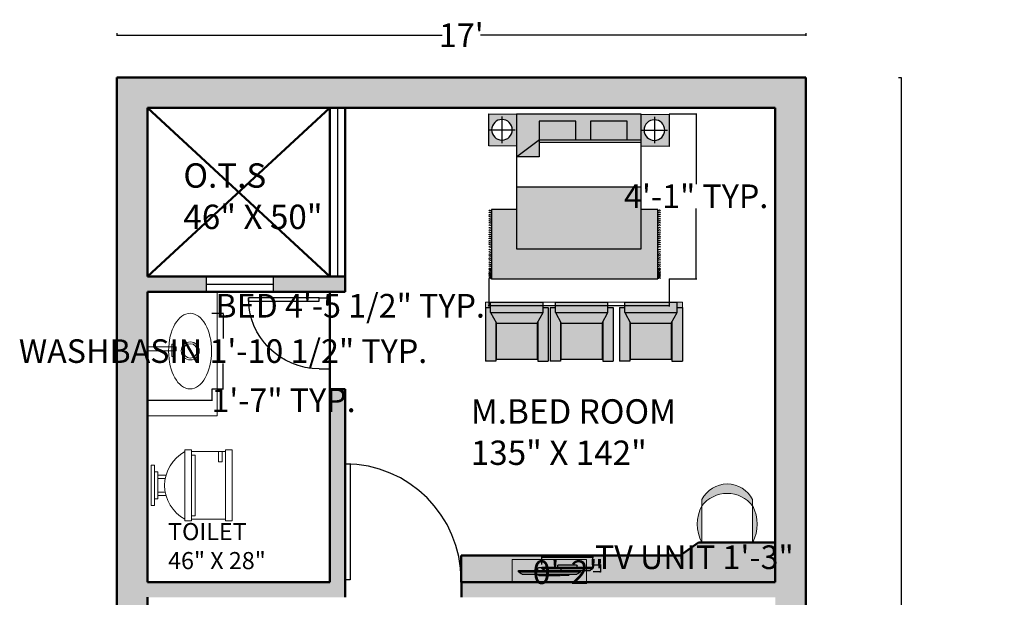
# Model space of a CAD drawing. Units: inches. Extents: x 679 to 1269, y 101 to 755.
# Tile 4 of 6: x 679 to 971, y 584 to 755. Entities that reach past the tile are written whole.
import ezdxf

# ---------------------------------------------------------------- set-up
doc = ezdxf.new("R2010")
doc.units = ezdxf.units.IN
doc.header["$MEASUREMENT"] = 0
for name, color, linetype, lineweight in [('A-ANNO-DIMS', 2, 'Continuous', 18), ('A-AREA-IDEN', 7, 'Continuous', 25), ('A-DOOR', 4, 'Continuous', 25), ('A-FLOR-FIXT', 8, 'Continuous', 18), ('A-FURN', 32, 'Continuous', 18), ('A-FURN-PATT', 252, 'Continuous', 13), ('A-GLAZ', 4, 'Continuous', 25), ('A-WALL', 7, 'Continuous', 50), ('A-WALL-PATT', 8, 'Continuous', 13)]:
    doc.layers.add(name, color=color, linetype=linetype, lineweight=lineweight)
doc.layers.add('furniture', color=32, linetype='Continuous')
doc.styles.get("Standard").update_dxf_attribs({"font": 'arial.ttf'})
doc.dimstyles.get("Standard").update_dxf_attribs({"dimtxt": 7, "dimasz": 0.18, "dimexe": 0.18, "dimexo": 0.0625, "dimgap": 0.09, "dimtad": 0, "dimtih": 1, "dimtoh": 1, "dimzin": 0, "dimdsep": 46, "dimlunit": 3, "dimtxsty": 'Standard', "dimcen": 0.09, "dimadec": 0, "dimazin": 0, "dimtfac": 1, "dimtofl": 0, "dimtmove": 0, "dimatfit": 3, "dimfxl": 1, "dimtolj": 1, "dimtzin": 0, "dimarcsym": 0})

# ---------------------------------------------------------------- blocks, each defined once
blk = doc.blocks.new('*D1')
at = {"layer": 'A-ANNO-DIMS', "color": 0, "lineweight": -2, "transparency": 16777216}
for p, q in [((708.21, 750.86), (708.21, 750.04)), ((708.39, 750.22), (804.51, 750.22)), ((912.03, 750.22), (815.91, 750.22)), ((912.21, 750.86), (912.21, 750.04))]:
    blk.add_line(p, q, dxfattribs=at)
at = {"layer": 'A-ANNO-DIMS', "color": 0, "transparency": 16777216}
for points in [[(708.39, 750.25), (708.39, 750.19), (708.21, 750.22)], [(912.03, 750.25), (912.03, 750.19), (912.21, 750.22)]]:
    blk.add_solid(points, dxfattribs=at)
at = {"layer": 'Defpoints', "color": 0, "transparency": 16777216}
for p in [(708.21, 750.92), (912.21, 750.92), (912.21, 750.22)]:
    blk.add_point(p, dxfattribs=at)
at = {"layer": 'A-ANNO-DIMS', "color": 0, "transparency": 16777216, "insert": (810.21, 750.22), "char_height": 7, "attachment_point": 5}
blk.add_mtext("\\A1;17'", dxfattribs=at)
blk = doc.blocks.new('*D2')
at = {"layer": 'A-ANNO-DIMS', "color": 0, "lineweight": -2, "transparency": 16777216}
for p, q in [((939.65, 737.73), (940.62, 737.73)), ((940.44, 737.55), (940.44, 441.39)), ((940.44, 137.91), (940.44, 434.07)), ((939.65, 137.73), (940.62, 137.73))]:
    blk.add_line(p, q, dxfattribs=at)
at = {"layer": 'A-ANNO-DIMS', "color": 0, "transparency": 16777216}
for points in [[(940.41, 737.55), (940.47, 737.55), (940.44, 737.73)], [(940.41, 137.91), (940.47, 137.91), (940.44, 137.73)]]:
    blk.add_solid(points, dxfattribs=at)
at = {"layer": 'Defpoints', "color": 0, "transparency": 16777216}
for p in [(939.59, 737.73), (939.59, 137.73), (940.44, 137.73)]:
    blk.add_point(p, dxfattribs=at)
at = {"layer": 'A-ANNO-DIMS', "color": 0, "transparency": 16777216, "insert": (940.44, 437.73), "char_height": 7, "attachment_point": 5}
blk.add_mtext("\\A1;50'", dxfattribs=at)
blk = doc.blocks.new('*U4')
for p, q in [((0, 0), (0, -6)), ((40, 0), (40, -6))]:
    blk.add_line(p, q)
blk.add_lwpolyline([(0, 0), (0, 40), (1.75, 40), (1.75, 0)], close=True)
blk.add_arc((0, 0), 40, 0, 90)
blk = doc.blocks.new('CARPET')
at = {"layer": 'furniture'}
for p, q in [((-51.53, -98.11), (-51.53, -55.12)), ((-51.53, -55.12), (-41.27, -55.12)), ((36, -55.12), (51.55, -55.12)), ((51.55, -55.12), (51.55, -98.11)), ((51.55, -98.11), (-51.53, -98.11))]:
    blk.add_line(p, q, dxfattribs=at)
for points, knots in [([(-53.37, -55.99), (-53.22, -55.8), (-52.9, -55.41), (-52.34, -55.8), (-51.89, -56.08), (-51.65, -55.91), (-51.53, -55.83)], [0, 0, 0, 0, 0.653278, 1.290138, 1.740457, 2.114451, 2.114451, 2.114451, 2.114451]), ([(-53.37, -57.26), (-53.22, -57.07), (-52.9, -56.67), (-52.34, -57.07), (-51.89, -57.35), (-51.65, -57.17), (-51.53, -57.1)], [0, 0, 0, 0, 0.653278, 1.290138, 1.740457, 2.114451, 2.114451, 2.114451, 2.114451]), ([(-53.37, -58.59), (-53.22, -58.4), (-52.9, -58.01), (-52.34, -58.4), (-51.89, -58.68), (-51.65, -58.5), (-51.53, -58.43)], [0, 0, 0, 0, 0.653278, 1.290138, 1.740457, 2.114451, 2.114451, 2.114451, 2.114451]), ([(-53.37, -59.78), (-53.22, -59.58), (-52.9, -59.19), (-52.34, -59.58), (-51.89, -59.86), (-51.65, -59.69), (-51.53, -59.61)], [0, 0, 0, 0, 0.653278, 1.290138, 1.740457, 2.114451, 2.114451, 2.114451, 2.114451]), ([(-53.37, -61.22), (-53.22, -61.02), (-52.9, -60.63), (-52.34, -61.02), (-51.89, -61.3), (-51.65, -61.13), (-51.53, -61.05)], [0, 0, 0, 0, 0.653278, 1.290138, 1.740457, 2.114451, 2.114451, 2.114451, 2.114451]), ([(53.37, -55.99), (53.22, -55.8), (52.9, -55.41), (52.34, -55.8), (51.89, -56.08), (51.65, -55.91), (51.53, -55.83)], [0, 0, 0, 0, 0.653278, 1.290138, 1.740457, 2.114451, 2.114451, 2.114451, 2.114451]), ([(53.37, -57.26), (53.22, -57.07), (52.9, -56.67), (52.34, -57.07), (51.89, -57.35), (51.65, -57.17), (51.53, -57.1)], [0, 0, 0, 0, 0.653278, 1.290138, 1.740457, 2.114451, 2.114451, 2.114451, 2.114451]), ([(53.37, -58.59), (53.22, -58.4), (52.9, -58.01), (52.34, -58.4), (51.89, -58.68), (51.65, -58.5), (51.53, -58.43)], [0, 0, 0, 0, 0.653278, 1.290138, 1.740457, 2.114451, 2.114451, 2.114451, 2.114451]), ([(53.37, -59.78), (53.22, -59.58), (52.9, -59.19), (52.34, -59.58), (51.89, -59.86), (51.65, -59.69), (51.53, -59.61)], [0, 0, 0, 0, 0.653278, 1.290138, 1.740457, 2.114451, 2.114451, 2.114451, 2.114451]), ([(53.37, -61.22), (53.22, -61.02), (52.9, -60.63), (52.34, -61.02), (51.89, -61.3), (51.65, -61.13), (51.53, -61.05)], [0, 0, 0, 0, 0.653278, 1.290138, 1.740457, 2.114451, 2.114451, 2.114451, 2.114451]), ([(-53.37, -62.44), (-53.22, -62.25), (-52.9, -61.86), (-52.34, -62.25), (-51.89, -62.53), (-51.65, -62.36), (-51.53, -62.28)], [0, 0, 0, 0, 0.653278, 1.290138, 1.740457, 2.114451, 2.114451, 2.114451, 2.114451]), ([(-53.37, -63.63), (-53.22, -63.43), (-52.9, -63.04), (-52.34, -63.43), (-51.89, -63.72), (-51.65, -63.54), (-51.53, -63.46)], [0, 0, 0, 0, 0.653278, 1.290138, 1.740457, 2.114451, 2.114451, 2.114451, 2.114451]), ([(-53.37, -65.07), (-53.22, -64.87), (-52.9, -64.48), (-52.34, -64.87), (-51.89, -65.15), (-51.65, -64.98), (-51.53, -64.9)], [0, 0, 0, 0, 0.653278, 1.290138, 1.740457, 2.114451, 2.114451, 2.114451, 2.114451]), ([(-53.37, -66.76), (-53.22, -66.56), (-52.9, -66.17), (-52.34, -66.56), (-51.89, -66.84), (-51.65, -66.67), (-51.53, -66.59)], [0, 0, 0, 0, 0.653278, 1.290138, 1.740457, 2.114451, 2.114451, 2.114451, 2.114451]), ([(53.37, -62.44), (53.22, -62.25), (52.9, -61.86), (52.34, -62.25), (51.89, -62.53), (51.65, -62.36), (51.53, -62.28)], [0, 0, 0, 0, 0.653278, 1.290138, 1.740457, 2.114451, 2.114451, 2.114451, 2.114451]), ([(53.37, -63.63), (53.22, -63.43), (52.9, -63.04), (52.34, -63.43), (51.89, -63.72), (51.65, -63.54), (51.53, -63.46)], [0, 0, 0, 0, 0.653278, 1.290138, 1.740457, 2.114451, 2.114451, 2.114451, 2.114451]), ([(53.37, -65.07), (53.22, -64.87), (52.9, -64.48), (52.34, -64.87), (51.89, -65.15), (51.65, -64.98), (51.53, -64.9)], [0, 0, 0, 0, 0.653278, 1.290138, 1.740457, 2.114451, 2.114451, 2.114451, 2.114451]), ([(53.37, -66.76), (53.22, -66.56), (52.9, -66.17), (52.34, -66.56), (51.89, -66.84), (51.65, -66.67), (51.53, -66.59)], [0, 0, 0, 0, 0.653278, 1.290138, 1.740457, 2.114451, 2.114451, 2.114451, 2.114451]), ([(-53.37, -68.2), (-53.22, -68), (-52.9, -67.61), (-52.34, -68), (-51.89, -68.28), (-51.65, -68.11), (-51.53, -68.03)], [0, 0, 0, 0, 0.653278, 1.290138, 1.740457, 2.114451, 2.114451, 2.114451, 2.114451]), ([(-53.37, -69.53), (-53.22, -69.33), (-52.9, -68.94), (-52.34, -69.33), (-51.89, -69.61), (-51.65, -69.44), (-51.53, -69.36)], [0, 0, 0, 0, 0.653278, 1.290138, 1.740457, 2.114451, 2.114451, 2.114451, 2.114451]), ([(-53.37, -70.79), (-53.22, -70.6), (-52.9, -70.21), (-52.34, -70.6), (-51.89, -70.88), (-51.65, -70.7), (-51.53, -70.63)], [0, 0, 0, 0, 0.653278, 1.290138, 1.740457, 2.114451, 2.114451, 2.114451, 2.114451]), ([(-53.37, -72.12), (-53.22, -71.93), (-52.9, -71.54), (-52.34, -71.93), (-51.89, -72.21), (-51.65, -72.04), (-51.53, -71.96)], [0, 0, 0, 0, 0.653278, 1.290138, 1.740457, 2.114451, 2.114451, 2.114451, 2.114451]), ([(-53.37, -73.31), (-53.22, -73.11), (-52.9, -72.72), (-52.34, -73.11), (-51.89, -73.4), (-51.65, -73.22), (-51.53, -73.14)], [0, 0, 0, 0, 0.653278, 1.290138, 1.740457, 2.114451, 2.114451, 2.114451, 2.114451]), ([(53.37, -68.2), (53.22, -68), (52.9, -67.61), (52.34, -68), (51.89, -68.28), (51.65, -68.11), (51.53, -68.03)], [0, 0, 0, 0, 0.653278, 1.290138, 1.740457, 2.114451, 2.114451, 2.114451, 2.114451]), ([(53.37, -69.53), (53.22, -69.33), (52.9, -68.94), (52.34, -69.33), (51.89, -69.61), (51.65, -69.44), (51.53, -69.36)], [0, 0, 0, 0, 0.653278, 1.290138, 1.740457, 2.114451, 2.114451, 2.114451, 2.114451]), ([(53.37, -70.79), (53.22, -70.6), (52.9, -70.21), (52.34, -70.6), (51.89, -70.88), (51.65, -70.7), (51.53, -70.63)], [0, 0, 0, 0, 0.653278, 1.290138, 1.740457, 2.114451, 2.114451, 2.114451, 2.114451]), ([(53.37, -72.12), (53.22, -71.93), (52.9, -71.54), (52.34, -71.93), (51.89, -72.21), (51.65, -72.04), (51.53, -71.96)], [0, 0, 0, 0, 0.653278, 1.290138, 1.740457, 2.114451, 2.114451, 2.114451, 2.114451]), ([(53.37, -73.31), (53.22, -73.11), (52.9, -72.72), (52.34, -73.11), (51.89, -73.4), (51.65, -73.22), (51.53, -73.14)], [0, 0, 0, 0, 0.653278, 1.290138, 1.740457, 2.114451, 2.114451, 2.114451, 2.114451]), ([(-53.37, -74.75), (-53.22, -74.55), (-52.9, -74.16), (-52.34, -74.55), (-51.89, -74.83), (-51.65, -74.66), (-51.53, -74.58)], [0, 0, 0, 0, 0.653278, 1.290138, 1.740457, 2.114451, 2.114451, 2.114451, 2.114451]), ([(-53.37, -75.98), (-53.22, -75.78), (-52.9, -75.39), (-52.34, -75.78), (-51.89, -76.06), (-51.65, -75.89), (-51.53, -75.81)], [0, 0, 0, 0, 0.653278, 1.290138, 1.740457, 2.114451, 2.114451, 2.114451, 2.114451]), ([(-53.37, -77.16), (-53.22, -76.96), (-52.9, -76.57), (-52.34, -76.96), (-51.89, -77.25), (-51.65, -77.07), (-51.53, -76.99)], [0, 0, 0, 0, 0.653278, 1.290138, 1.740457, 2.114451, 2.114451, 2.114451, 2.114451]), ([(-53.37, -78.6), (-53.22, -78.4), (-52.9, -78.01), (-52.34, -78.4), (-51.89, -78.68), (-51.65, -78.51), (-51.53, -78.43)], [0, 0, 0, 0, 0.653278, 1.290138, 1.740457, 2.114451, 2.114451, 2.114451, 2.114451]), ([(53.37, -74.75), (53.22, -74.55), (52.9, -74.16), (52.34, -74.55), (51.89, -74.83), (51.65, -74.66), (51.53, -74.58)], [0, 0, 0, 0, 0.653278, 1.290138, 1.740457, 2.114451, 2.114451, 2.114451, 2.114451]), ([(53.37, -75.98), (53.22, -75.78), (52.9, -75.39), (52.34, -75.78), (51.89, -76.06), (51.65, -75.89), (51.53, -75.81)], [0, 0, 0, 0, 0.653278, 1.290138, 1.740457, 2.114451, 2.114451, 2.114451, 2.114451]), ([(53.37, -77.16), (53.22, -76.96), (52.9, -76.57), (52.34, -76.96), (51.89, -77.25), (51.65, -77.07), (51.53, -76.99)], [0, 0, 0, 0, 0.653278, 1.290138, 1.740457, 2.114451, 2.114451, 2.114451, 2.114451]), ([(53.37, -78.6), (53.22, -78.4), (52.9, -78.01), (52.34, -78.4), (51.89, -78.68), (51.65, -78.51), (51.53, -78.43)], [0, 0, 0, 0, 0.653278, 1.290138, 1.740457, 2.114451, 2.114451, 2.114451, 2.114451]), ([(-53.37, -80.29), (-53.22, -80.09), (-52.9, -79.7), (-52.34, -80.09), (-51.89, -80.37), (-51.65, -80.2), (-51.53, -80.12)], [0, 0, 0, 0, 0.653278, 1.290138, 1.740457, 2.114451, 2.114451, 2.114451, 2.114451]), ([(-53.37, -81.73), (-53.22, -81.53), (-52.9, -81.14), (-52.34, -81.53), (-51.89, -81.81), (-51.65, -81.64), (-51.53, -81.56)], [0, 0, 0, 0, 0.653278, 1.290138, 1.740457, 2.114451, 2.114451, 2.114451, 2.114451]), ([(-53.37, -83.06), (-53.22, -82.86), (-52.9, -82.47), (-52.34, -82.86), (-51.89, -83.14), (-51.65, -82.97), (-51.53, -82.89)], [0, 0, 0, 0, 0.653278, 1.290138, 1.740457, 2.114451, 2.114451, 2.114451, 2.114451]), ([(-53.37, -84.18), (-53.22, -83.99), (-52.9, -83.6), (-52.34, -83.99), (-51.89, -84.27), (-51.65, -84.09), (-51.53, -84.02)], [0, 0, 0, 0, 0.653278, 1.290138, 1.740457, 2.114451, 2.114451, 2.114451, 2.114451]), ([(-53.37, -85.51), (-53.22, -85.32), (-52.9, -84.93), (-52.34, -85.32), (-51.89, -85.6), (-51.65, -85.42), (-51.53, -85.35)], [0, 0, 0, 0, 0.653278, 1.290138, 1.740457, 2.114451, 2.114451, 2.114451, 2.114451]), ([(53.37, -80.29), (53.22, -80.09), (52.9, -79.7), (52.34, -80.09), (51.89, -80.37), (51.65, -80.2), (51.53, -80.12)], [0, 0, 0, 0, 0.653278, 1.290138, 1.740457, 2.114451, 2.114451, 2.114451, 2.114451]), ([(53.37, -81.73), (53.22, -81.53), (52.9, -81.14), (52.34, -81.53), (51.89, -81.81), (51.65, -81.64), (51.53, -81.56)], [0, 0, 0, 0, 0.653278, 1.290138, 1.740457, 2.114451, 2.114451, 2.114451, 2.114451]), ([(53.37, -83.06), (53.22, -82.86), (52.9, -82.47), (52.34, -82.86), (51.89, -83.14), (51.65, -82.97), (51.53, -82.89)], [0, 0, 0, 0, 0.653278, 1.290138, 1.740457, 2.114451, 2.114451, 2.114451, 2.114451]), ([(53.37, -84.18), (53.22, -83.99), (52.9, -83.6), (52.34, -83.99), (51.89, -84.27), (51.65, -84.09), (51.53, -84.02)], [0, 0, 0, 0, 0.653278, 1.290138, 1.740457, 2.114451, 2.114451, 2.114451, 2.114451]), ([(53.37, -85.51), (53.22, -85.32), (52.9, -84.93), (52.34, -85.32), (51.89, -85.6), (51.65, -85.42), (51.53, -85.35)], [0, 0, 0, 0, 0.653278, 1.290138, 1.740457, 2.114451, 2.114451, 2.114451, 2.114451]), ([(-53.37, -86.7), (-53.22, -86.5), (-52.9, -86.11), (-52.34, -86.5), (-51.89, -86.78), (-51.65, -86.61), (-51.53, -86.53)], [0, 0, 0, 0, 0.653278, 1.290138, 1.740457, 2.114451, 2.114451, 2.114451, 2.114451]), ([(-53.37, -88.14), (-53.22, -87.94), (-52.9, -87.55), (-52.34, -87.94), (-51.89, -88.22), (-51.65, -88.05), (-51.53, -87.97)], [0, 0, 0, 0, 0.653278, 1.290138, 1.740457, 2.114451, 2.114451, 2.114451, 2.114451]), ([(-53.37, -89.36), (-53.22, -89.17), (-52.9, -88.78), (-52.34, -89.17), (-51.89, -89.45), (-51.65, -89.28), (-51.53, -89.2)], [0, 0, 0, 0, 0.653278, 1.290138, 1.740457, 2.114451, 2.114451, 2.114451, 2.114451]), ([(-53.37, -90.55), (-53.22, -90.35), (-52.9, -89.96), (-52.34, -90.35), (-51.89, -90.64), (-51.65, -90.46), (-51.53, -90.38)], [0, 0, 0, 0, 0.653278, 1.290138, 1.740457, 2.114451, 2.114451, 2.114451, 2.114451]), ([(-53.37, -91.99), (-53.22, -91.79), (-52.9, -91.4), (-52.34, -91.79), (-51.89, -92.07), (-51.65, -91.9), (-51.53, -91.82)], [0, 0, 0, 0, 0.653278, 1.290138, 1.740457, 2.114451, 2.114451, 2.114451, 2.114451]), ([(53.37, -86.7), (53.22, -86.5), (52.9, -86.11), (52.34, -86.5), (51.89, -86.78), (51.65, -86.61), (51.53, -86.53)], [0, 0, 0, 0, 0.653278, 1.290138, 1.740457, 2.114451, 2.114451, 2.114451, 2.114451]), ([(53.37, -88.14), (53.22, -87.94), (52.9, -87.55), (52.34, -87.94), (51.89, -88.22), (51.65, -88.05), (51.53, -87.97)], [0, 0, 0, 0, 0.653278, 1.290138, 1.740457, 2.114451, 2.114451, 2.114451, 2.114451]), ([(53.37, -89.36), (53.22, -89.17), (52.9, -88.78), (52.34, -89.17), (51.89, -89.45), (51.65, -89.28), (51.53, -89.2)], [0, 0, 0, 0, 0.653278, 1.290138, 1.740457, 2.114451, 2.114451, 2.114451, 2.114451]), ([(53.37, -90.55), (53.22, -90.35), (52.9, -89.96), (52.34, -90.35), (51.9, -90.63), (51.66, -90.47), (51.55, -90.4)], [0, 0, 0, 0, 0.653278, 1.290138, 1.740457, 2.0926, 2.0926, 2.0926, 2.0926]), ([(53.37, -91.99), (53.22, -91.79), (52.9, -91.4), (52.34, -91.79), (51.9, -92.07), (51.66, -91.91), (51.55, -91.83)], [0, 0, 0, 0, 0.653278, 1.290138, 1.740457, 2.0926, 2.0926, 2.0926, 2.0926]), ([(-53.37, -92.69), (-53.22, -92.48), (-52.9, -92.08), (-52.35, -92.49), (-51.89, -92.77), (-51.65, -92.6), (-51.53, -92.52)], [0, 0, 0, 0, 0.663904, 1.307406, 1.757725, 2.131719, 2.131719, 2.131719, 2.131719]), ([(-53.37, -93.61), (-53.22, -93.42), (-52.9, -93.03), (-52.34, -93.42), (-51.89, -93.7), (-51.65, -93.52), (-51.53, -93.45)], [0, 0, 0, 0, 0.653278, 1.290138, 1.740457, 2.114451, 2.114451, 2.114451, 2.114451]), ([(-53.37, -94.55), (-53.22, -94.35), (-52.9, -93.96), (-52.34, -94.35), (-51.89, -94.63), (-51.65, -94.46), (-51.53, -94.38)], [0, 0, 0, 0, 0.653278, 1.290138, 1.740457, 2.114451, 2.114451, 2.114451, 2.114451]), ([(-53.37, -95.05), (-53.22, -94.85), (-52.9, -94.46), (-52.34, -94.85), (-51.89, -95.14), (-51.65, -94.96), (-51.53, -94.88)], [0, 0, 0, 0, 0.653278, 1.290138, 1.740457, 2.114451, 2.114451, 2.114451, 2.114451]), ([(-53.37, -95.73), (-53.22, -95.54), (-52.9, -95.15), (-52.34, -95.54), (-51.89, -95.82), (-51.65, -95.65), (-51.53, -95.57)], [0, 0, 0, 0, 0.653278, 1.290138, 1.740457, 2.114451, 2.114451, 2.114451, 2.114451]), ([(-53.37, -96.38), (-53.22, -96.18), (-52.9, -95.79), (-52.34, -96.18), (-51.89, -96.47), (-51.65, -96.29), (-51.53, -96.21)], [0, 0, 0, 0, 0.653278, 1.290138, 1.740457, 2.114451, 2.114451, 2.114451, 2.114451]), ([(-53.37, -97.17), (-53.22, -96.98), (-52.9, -96.59), (-52.34, -96.98), (-51.89, -97.26), (-51.65, -97.08), (-51.53, -97.01)], [0, 0, 0, 0, 0.653278, 1.290138, 1.740457, 2.114451, 2.114451, 2.114451, 2.114451]), ([(-53.37, -97.99), (-53.22, -97.79), (-52.9, -97.4), (-52.34, -97.79), (-51.89, -98.08), (-51.65, -97.9), (-51.53, -97.82)], [0, 0, 0, 0, 0.653278, 1.290138, 1.740457, 2.114451, 2.114451, 2.114451, 2.114451]), ([(53.37, -95.78), (53.22, -95.58), (52.9, -95.19), (52.34, -95.58), (51.89, -95.86), (51.65, -95.69), (51.53, -95.61)], [0, 0, 0, 0, 0.653278, 1.290138, 1.740457, 2.114451, 2.114451, 2.114451, 2.114451]), ([(53.37, -96.43), (53.22, -96.23), (52.9, -95.84), (52.34, -96.23), (51.89, -96.51), (51.65, -96.34), (51.53, -96.26)], [0, 0, 0, 0, 0.653278, 1.290138, 1.740457, 2.114451, 2.114451, 2.114451, 2.114451]), ([(53.37, -97.22), (53.22, -97.02), (52.9, -96.63), (52.34, -97.02), (51.89, -97.3), (51.65, -97.13), (51.53, -97.05)], [0, 0, 0, 0, 0.653278, 1.290138, 1.740457, 2.114451, 2.114451, 2.114451, 2.114451]), ([(53.37, -97.99), (53.22, -97.79), (52.9, -97.4), (52.34, -97.79), (51.89, -98.08), (51.65, -97.9), (51.53, -97.82)], [0, 0, 0, 0, 0.653278, 1.290138, 1.740457, 2.114451, 2.114451, 2.114451, 2.114451]), ([(53.37, -92.69), (53.22, -92.49), (52.9, -92.09), (52.34, -92.49), (51.9, -92.77), (51.66, -92.61), (51.55, -92.53)], [0, 0, 0, 0, 0.656792, 1.295826, 1.746145, 2.098292, 2.098292, 2.098292, 2.098292]), ([(53.37, -93.66), (53.22, -93.46), (52.9, -93.07), (52.34, -93.46), (51.9, -93.74), (51.66, -93.58), (51.55, -93.5)], [0, 0, 0, 0, 0.653278, 1.290138, 1.740457, 2.0926, 2.0926, 2.0926, 2.0926]), ([(53.37, -94.59), (53.22, -94.4), (52.9, -94.01), (52.34, -94.4), (51.9, -94.68), (51.66, -94.51), (51.55, -94.44)], [0, 0, 0, 0, 0.653278, 1.290138, 1.740457, 2.0926, 2.0926, 2.0926, 2.0926]), ([(53.37, -95.1), (53.22, -94.9), (52.9, -94.51), (52.34, -94.9), (51.9, -95.18), (51.66, -95.02), (51.55, -94.94)], [0, 0, 0, 0, 0.653278, 1.290138, 1.740457, 2.0926, 2.0926, 2.0926, 2.0926])]:
    blk.add_open_spline(points, degree=3, knots=knots, dxfattribs=at)
blk = doc.blocks.new('A$C58D270C6')
at = {"layer": 'furniture'}
for p, q in [((9.09, 124.13), (9.09, 108.87)), ((1.46, 116.5), (16.73, 116.5)), ((14.97, 94.84), (24.62, 107.92)), ((24.62, 94.93), (24.62, 107.92)), ((42.08, 108), (42.08, 36)), ((14.97, 94.93), (24.62, 94.93)), ((14.97, 94.84), (14.97, 36)), ((16.22, 94.93), (16.22, 36)), ((9.25, 36), (9.25, 20.74)), ((1.62, 28.37), (16.88, 28.37))]:
    blk.add_line(p, q, dxfattribs=at)
for points in [[(18.5, 108), (18.34, 124.13), (-0.16, 124.13), (0, 108)], [(0, 108), (77.91, 108), (77.91, 36), (0, 36)], [(4.09, 94.93), (14.97, 94.93), (14.97, 73.83), (4.09, 73.83)], [(4.09, 65.23), (14.97, 65.23), (14.97, 44.13), (4.09, 44.13)], [(18.65, 19.87), (18.5, 36), (0, 36), (0.16, 19.87)]]:
    blk.add_lwpolyline(points, close=True, dxfattribs=at)
for centre in [(9.09, 116.5), (9.25, 28.37)]:
    blk.add_circle(centre, 5.95, dxfattribs=at)
at = {"layer": 'furniture', "xscale": 0.9312884925094044, "yscale": 0.9312884925094044, "zscale": 0.9312884925094044, "rotation": 90}
blk.add_blockref('CARPET', (3.79, 74.47), dxfattribs=at)
blk = doc.blocks.new('FABRIC SOFA 1S')
at = {"layer": 'furniture'}
for p, q in [((3, 18.12), (34, 18.12)), ((3, 15.12), (3, 18.12)), ((34, 12.12), (34, 18.12)), ((0, -15.12), (0, 15.12)), ((6, 15.12), (0, 15.12)), ((6, -15.12), (6, 15.12)), ((12, 11.75), (6, 15.12)), ((11.33, 12.12), (34, 12.12)), ((6, -15.12), (0, -15.12)), ((3, -18.12), (3, -15.12)), ((6, -15.12), (12, -11.75)), ((11.33, -12.12), (34, -12.12)), ((34, -12.12), (34, -18.12)), ((3, -18.12), (34, -18.12))]:
    blk.add_line(p, q, dxfattribs=at)
blk.add_lwpolyline([(12, -11.75), (12, 11.75), (33, 11.75), (33, -11.75)], close=True, dxfattribs=at)
blk = doc.blocks.new('*U12')
for p, q in [((-10, 22), (-10, 12)), ((-10, 21), (-7, 21)), ((-7, 21), (-7, 20)), ((10, 12), (10, 22)), ((-7, 20), (-10, 20)), ((10.5, 12), (-10.5, 12)), ((-10.5, 10), (-10.5, 12)), ((9, 13), (-9, 13)), ((-9, 13), (-9, 12)), ((9, 12), (9, 13)), ((10.5, 12), (10.5, 10)), ((10.5, 10), (-10.5, 10)), ((-3, 4.4065), (-3, 2)), ((-2, 2), (-2, 4.1658)), ((2, 4.1658), (2, 2)), ((3, 2), (3, 4.4065)), ((4, 2), (-4, 2)), ((-4, 2), (-4, 1)), ((4, 1), (4, 2))]:
    blk.add_line(p, q)
for points in [[(10.5, 22), (10.5, 24), (-10.5, 24), (-10.5, 22)], [(6, 0), (6, 1), (-6, 1), (-6, 0)]]:
    blk.add_lwpolyline(points, close=True)
blk.add_arc((0, 15.3333), 11.3333, 208.0725, 331.9275)
blk = doc.blocks.new('PLASMA-LARGE')
at = {"layer": 'furniture'}
for p, q in [((-7.26, 0), (7.26, 0)), ((-21, -2.5), (21, -2.5)), ((-21, -2.5), (-21, -3.5)), ((-21, -3.5), (21, -3.5)), ((-18.61, -1), (18.61, -1)), ((-8, -1), (-8, -0.74)), ((-8, -3.5), (-8, -4.76)), ((-7.26, -5.5), (7.26, -5.5)), ((8, -1), (8, -0.74)), ((8, -3.5), (8, -4.76)), ((21, -2.5), (21, -3.5))]:
    blk.add_line(p, q, dxfattribs=at)
for centre, radius, start, end in [((-7.26, -0.74), 0.744, 90, 180), ((7.26, -0.74), 0.744, 0, 90), ((-13.97, -11.05), 11.07, 114.76019, 129.41749), ((-7.26, -4.76), 0.744, 180, 270), ((7.26, -4.76), 0.744, 270, 0), ((13.97, -11.05), 11.07, 50.58251, 65.23981)]:
    blk.add_arc(centre, radius, start, end, dxfattribs=at)
blk = doc.blocks.new('WASHBASIN')
for p, q in [((8.57, 12.49), (0, 12.49)), ((7.24, 9.62), (7.23, 13.28)), ((7.23, 13.28), (7.63, 13.28)), ((7.63, 13.28), (7.65, 9.63)), ((8.57, 11.25), (8.57, 12.49)), ((8.57, 11.25), (0, 11.25)), ((7.24, 9.62), (7.65, 9.63))]:
    blk.add_line(p, q)
for radius in [2.67, 2.13]:
    blk.add_circle((12.7, 11.27), radius)
at = {"extrusion": (0, 0, -1)}
blk.add_ellipse((12.66, 11.2), major_axis=(0.03, 11.2), ratio=0.56899, dxfattribs=at)
blk = doc.blocks.new('CHAIR')
h = blk.add_hatch(color=256)
h.dxf.hatch_style = 1
h.paths.add_polyline_path([(1.35, 12.72), (1.35, 10.82, -0.490483), (16.4, 10.82), (16.4, 12.72, 0.611129)])
h.paths.add_polyline_path([(1.35, 10.82, 0.248963), (1.35, 0)])
h.paths.add_polyline_path([(16.4, 10.82), (16.4, 0, 0.248963)])
for p, q in [((1.35, 12.72), (1.35, 0)), ((16.4, 12.72), (16.4, 0))]:
    blk.add_line(p, q)
for centre, radius, start, end in [((8.87, 8.86), 8.46, 27.1394, 152.8606), ((8.87, 4.99), 9.52, 37.7457, 142.2543), ((11.54, 5.41), 11.54, 152.0394, 207.9606), ((6.21, 5.41), 11.54, 332.0394, 27.9606)]:
    blk.add_arc(centre, radius, start, end)
blk = doc.blocks.new('*D21')
at = {"layer": 'A-ANNO-DIMS', "color": 0, "lineweight": -2, "transparency": 16777216}
for p, q in [((818.31, 678.03), (818.31, 669.9)), ((871.75, 678.03), (871.75, 669.9)), ((818.31, 670.08), (818.13, 670.08)), ((871.57, 670.08), (818.49, 670.08))]:
    blk.add_line(p, q, dxfattribs=at)
at = {"layer": 'A-ANNO-DIMS', "color": 0, "transparency": 16777216}
for points in [[(818.49, 670.11), (818.49, 670.05), (818.31, 670.08)], [(871.57, 670.11), (871.57, 670.05), (871.75, 670.08)]]:
    blk.add_solid(points, dxfattribs=at)
at = {"layer": 'Defpoints', "color": 0, "transparency": 16777216}
for p in [(818.31, 678.1), (871.75, 678.1), (818.31, 670.08)]:
    blk.add_point(p, dxfattribs=at)
at = {"layer": 'A-ANNO-DIMS', "color": 0, "transparency": 16777216, "insert": (777.29, 670.08), "char_height": 7, "attachment_point": 5}
blk.add_mtext('\\A1;BED 4\'-5 1/2" TYP.', dxfattribs=at)
blk = doc.blocks.new('*D22')
at = {"layer": 'A-ANNO-DIMS', "color": 0, "lineweight": -2, "transparency": 16777216}
for p, q in [((871.81, 726.93), (879.95, 726.93)), ((879.77, 726.75), (879.77, 706.12)), ((879.77, 678.28), (879.77, 698.91)), ((871.81, 678.1), (879.95, 678.1))]:
    blk.add_line(p, q, dxfattribs=at)
at = {"layer": 'A-ANNO-DIMS', "color": 0, "transparency": 16777216}
for points in [[(879.74, 726.75), (879.8, 726.75), (879.77, 726.93)], [(879.74, 678.28), (879.8, 678.28), (879.77, 678.1)]]:
    blk.add_solid(points, dxfattribs=at)
at = {"layer": 'Defpoints', "color": 0, "transparency": 16777216}
for p in [(871.75, 726.93), (871.75, 678.1), (879.77, 678.1)]:
    blk.add_point(p, dxfattribs=at)
at = {"layer": 'A-ANNO-DIMS', "color": 0, "transparency": 16777216, "insert": (879.77, 702.51), "char_height": 7, "attachment_point": 5}
blk.add_mtext('\\A1;4\'-1" TYP.', dxfattribs=at)
blk = doc.blocks.new('*D31')
at = {"layer": 'A-ANNO-DIMS', "color": 0, "lineweight": -2, "transparency": 16777216}
for p, q in [((834.08, 593.4), (834.08, 595.78)), ((834.26, 595.6), (849.02, 595.6)), ((849.2, 593.4), (849.2, 595.78)), ((849.2, 595.6), (849.38, 595.6))]:
    blk.add_line(p, q, dxfattribs=at)
at = {"layer": 'A-ANNO-DIMS', "color": 0, "transparency": 16777216}
for points in [[(834.26, 595.63), (834.26, 595.57), (834.08, 595.6)], [(849.02, 595.63), (849.02, 595.57), (849.2, 595.6)]]:
    blk.add_solid(points, dxfattribs=at)
at = {"layer": 'Defpoints', "color": 0, "transparency": 16777216}
for p in [(849.2, 595.6), (834.08, 593.34), (849.2, 593.34)]:
    blk.add_point(p, dxfattribs=at)
at = {"layer": 'A-ANNO-DIMS', "color": 0, "transparency": 16777216, "insert": (879.23, 595.6), "char_height": 7, "attachment_point": 5}
blk.add_mtext('\\A1;TV UNIT 1\'-3"', dxfattribs=at)
blk = doc.blocks.new('*D32')
at = {"layer": 'A-ANNO-DIMS', "color": 0, "lineweight": -2, "transparency": 16777216}
for p, q in [((849.26, 593.34), (851.64, 593.34)), ((851.46, 593.16), (851.46, 591.54)), ((849.26, 591.36), (851.64, 591.36)), ((851.46, 591.18), (851.28, 591.18)), ((851.46, 591.36), (851.46, 591.18))]:
    blk.add_line(p, q, dxfattribs=at)
at = {"layer": 'A-ANNO-DIMS', "color": 0, "transparency": 16777216}
for points in [[(851.43, 593.16), (851.49, 593.16), (851.46, 593.34)], [(851.43, 591.54), (851.49, 591.54), (851.46, 591.36)]]:
    blk.add_solid(points, dxfattribs=at)
at = {"layer": 'Defpoints', "color": 0, "transparency": 16777216}
for p in [(849.2, 593.34), (849.2, 591.36), (851.46, 591.36)]:
    blk.add_point(p, dxfattribs=at)
at = {"layer": 'A-ANNO-DIMS', "color": 0, "transparency": 16777216, "insert": (841.89, 591.18), "char_height": 7, "attachment_point": 5}
blk.add_mtext('\\A1;0\'-2"', dxfattribs=at)
blk = doc.blocks.new('*D37')
at = {"layer": 'A-ANNO-DIMS', "color": 0, "lineweight": -2, "transparency": 16777216}
for p, q in [((736.33, 667.87), (739.81, 667.87)), ((739.63, 667.69), (739.63, 660.36)), ((739.63, 645.62), (739.63, 652.94)), ((736.33, 645.44), (739.81, 645.44))]:
    blk.add_line(p, q, dxfattribs=at)
at = {"layer": 'A-ANNO-DIMS', "color": 0, "transparency": 16777216}
for points in [[(739.6, 667.69), (739.66, 667.69), (739.63, 667.87)], [(739.6, 645.62), (739.66, 645.62), (739.63, 645.44)]]:
    blk.add_solid(points, dxfattribs=at)
at = {"layer": 'Defpoints', "color": 0, "transparency": 16777216}
for p in [(736.26, 667.87), (739.63, 667.87), (736.26, 645.44)]:
    blk.add_point(p, dxfattribs=at)
at = {"layer": 'A-ANNO-DIMS', "color": 0, "transparency": 16777216, "insert": (739.63, 656.65), "char_height": 7, "attachment_point": 5}
blk.add_mtext('\\A1;WASHBASIN 1\'-10 1/2" TYP.', dxfattribs=at)
blk = doc.blocks.new('*D38')
at = {"layer": 'A-ANNO-DIMS', "color": 0, "lineweight": -2, "transparency": 16777216}
for p, q in [((717.21, 645.38), (717.21, 641.9)), ((736.26, 645.38), (736.26, 641.9)), ((717.39, 642.08), (736.08, 642.08)), ((736.26, 642.08), (736.44, 642.08))]:
    blk.add_line(p, q, dxfattribs=at)
at = {"layer": 'A-ANNO-DIMS', "color": 0, "transparency": 16777216}
for points in [[(717.39, 642.11), (717.39, 642.05), (717.21, 642.08)], [(736.08, 642.11), (736.08, 642.05), (736.26, 642.08)]]:
    blk.add_solid(points, dxfattribs=at)
at = {"layer": 'Defpoints', "color": 0, "transparency": 16777216}
for p in [(717.21, 645.44), (736.26, 645.44), (736.26, 642.08)]:
    blk.add_point(p, dxfattribs=at)
at = {"layer": 'A-ANNO-DIMS', "color": 0, "transparency": 16777216, "insert": (757.54, 642.08), "char_height": 7, "attachment_point": 5}
blk.add_mtext('\\A1;1\'-7" TYP.', dxfattribs=at)

msp = doc.modelspace()

# ---------------------------------------------------------------- hatches: boundary and pattern name
at = {"layer": 'A-FURN-PATT'}
h = msp.add_hatch(color=256, dxfattribs=at)
h.dxf.hatch_style = 1
h.paths.add_polyline_path([(834.431, 671.141), (818.876, 671.141), (818.876, 668.056), (834.431, 668.056)])
h.paths.add_polyline_path([(834.431, 668.056), (818.876, 668.056), (820.611, 664.971), (832.695, 664.971)])
h.paths.add_polyline_path([(820.418, 665.313), (818.876, 668.056), (818.876, 669.599), (817.333, 669.599), (817.333, 653.658), (820.418, 653.658)])
h.paths.add_polyline_path([(832.695, 664.971), (820.611, 664.971), (820.611, 654.172), (832.695, 654.172)])
h.paths.add_polyline_path([(835.973, 669.599), (834.431, 669.599), (834.431, 668.056), (832.888, 665.313), (832.888, 653.658), (835.973, 653.658)])
h.paths.add_polyline_path([(818.876, 671.141), (817.333, 671.141), (817.333, 669.599), (818.876, 669.599)])
h = msp.add_hatch(color=256, dxfattribs=at)
h.dxf.hatch_style = 1
h.paths.add_polyline_path([(853.639, 671.141), (838.084, 671.141), (838.084, 668.056), (853.639, 668.056)])
h.paths.add_polyline_path([(853.639, 668.056), (838.084, 668.056), (839.819, 664.971), (851.904, 664.971)])
h.paths.add_polyline_path([(839.627, 665.313), (838.084, 668.056), (838.084, 669.599), (836.541, 669.599), (836.541, 653.658), (839.627, 653.658)])
h.paths.add_polyline_path([(855.182, 669.599), (853.639, 669.599), (853.639, 668.056), (852.096, 665.313), (852.096, 653.658), (855.182, 653.658)])
h.paths.add_polyline_path([(851.904, 664.971), (839.819, 664.971), (839.819, 654.172), (851.904, 654.172)])
h = msp.add_hatch(color=256, dxfattribs=at)
h.dxf.hatch_style = 1
h.paths.add_polyline_path([(874.146, 671.141), (858.591, 671.141), (858.591, 668.056), (874.146, 668.056)])
h.paths.add_polyline_path([(874.146, 668.056), (858.591, 668.056), (860.326, 664.971), (872.41, 664.971)])
h.paths.add_polyline_path([(860.133, 665.313), (858.591, 668.056), (858.591, 669.599), (857.048, 669.599), (857.048, 653.658), (860.133, 653.658)])
h.paths.add_polyline_path([(872.41, 664.971), (860.326, 664.971), (860.326, 654.172), (872.41, 654.172)])
h.paths.add_polyline_path([(875.689, 669.599), (874.146, 669.599), (874.146, 668.056), (872.603, 665.313), (872.603, 653.658), (875.689, 653.658)])
h.paths.add_polyline_path([(875.689, 671.141), (874.146, 671.141), (874.146, 669.599), (875.689, 669.599)])
h = msp.add_hatch(color=256, dxfattribs=at)
h.dxf.hatch_style = 1
h.paths.add_polyline_path([(903.214, 599.984), (880.455, 599.984), (875.045, 596.11), (810.145, 596.11), (810.145, 588.883), (810.145, 588.229), (903.214, 588.229)])
h = msp.add_hatch(color=256, dxfattribs=at)
h.dxf.hatch_style = 1
h.paths.add_polyline_path([(847.257, 594.975), (825.239, 594.975), (825.239, 588.229), (847.257, 588.229)])
h.paths.add_polyline_path([(832.834, 591.674), (832.834, 592.223, -0.4142136), (833.159, 592.548), (839.504, 592.548, -0.4142136), (839.829, 592.223), (839.829, 591.674), (845.512, 591.674), (845.512, 591.237, -0.0640419), (844.466, 590.581), (839.829, 590.581), (839.829, 590.469, -0.4142136), (839.504, 590.144), (833.159, 590.144, -0.4142136), (832.834, 590.469), (832.834, 590.581), (828.197, 590.581, -0.0640419), (827.151, 591.237), (827.151, 591.674)], flags=16)
at = {"layer": 'A-WALL-PATT'}
h = msp.add_hatch(color=256, dxfattribs=at)
h.dxf.hatch_style = 1
h.paths.add_polyline_path([(775.786, 535.729), (771.286, 535.729), (771.286, 454.229), (717.214, 454.229), (717.214, 531.229), (742.559, 531.229), (742.559, 535.729), (717.214, 535.729), (717.214, 583.729), (775.786, 583.729), (775.786, 588.883), (775.786, 623.243), (775.786, 645.329), (771.286, 645.329), (771.286, 588.229), (717.214, 588.229), (717.214, 674.229), (734.589, 674.229), (734.589, 678.729), (717.214, 678.729), (717.214, 728.729), (903.214, 728.729), (903.214, 588.229), (810.214, 588.229), (810.214, 583.729), (903.214, 583.729), (903.214, 374.229), (851.714, 374.229), (851.714, 369.729), (903.214, 369.729), (903.214, 312.729), (856.214, 312.729), (856.214, 341.229), (851.714, 341.229), (851.714, 308.229), (903.214, 308.229), (903.214, 137.729), (912.214, 137.729), (912.214, 737.729), (708.214, 737.729), (708.214, 137.729), (717.214, 137.729), (717.214, 197.763), (776.196, 197.763), (776.196, 202.263), (717.214, 202.263), (717.214, 449.729), (771.286, 449.729), (771.286, 350.298), (775.786, 350.298), (775.786, 531.229)])
h = msp.add_hatch(color=256, dxfattribs=at)
h.dxf.hatch_style = 1
h.paths.add_polyline_path([(1180.931, 507.268), (1089.362, 507.268), (1089.362, 356.354), (1180.931, 356.354)])
h.paths.add_polyline_path([(1037.949, 416.536), (999.347, 416.536), (999.347, 387.67), (1037.949, 387.67)])
h.paths.add_polyline_path([(1037.949, 579.213), (999.347, 579.213), (999.347, 550.347), (1037.949, 550.347)])
h.paths.add_polyline_path([(1064.382, 465.7), (1050.613, 465.7), (1050.613, 440.519), (1064.382, 440.519)])
h.paths.add_polyline_path([(1064.382, 534.011), (1050.613, 534.011), (1050.613, 508.83), (1064.382, 508.83)])
h.paths.add_polyline_path([(1017.114, 194.268), (1003.506, 194.268), (1003.391, 182.402), (1010.195, 182.402), (1010.195, 183.635, -0.4142136), (1005.815, 188.015, -1), (1014.576, 188.015, -0.4142136), (1010.195, 183.635), (1010.195, 182.402), (1017, 182.402)])
h.paths.add_polyline_path([(1014.691, 252.849, -0.4142136), (1010.31, 248.468), (1010.31, 247.235), (1017.114, 247.235), (1017.229, 259.102), (1003.62, 259.102), (1003.506, 247.235), (1010.31, 247.235), (1010.31, 248.468, -0.4142136), (1005.929, 252.849, -1)])
h.paths.add_polyline_path([(1104.314, 726.852), (1096.049, 726.931), (1096.049, 722.192), (1096.908, 722.192, -1), (1103.01, 722.192, -1), (1096.908, 722.192), (1096.049, 722.192), (1096.049, 717.453), (1104.314, 717.374)])
h.paths.add_polyline_path([(1149.469, 726.772), (1141.204, 726.852), (1141.204, 722.113), (1142.063, 722.113, -1), (1148.165, 722.113, -1), (1142.063, 722.113), (1141.204, 722.113), (1141.204, 717.374), (1149.469, 717.294)])
h.paths.add_polyline_path([(826.598, 726.852), (818.333, 726.931), (818.333, 722.192), (819.192, 722.192, -1), (825.294, 722.192, -1), (819.192, 722.192), (818.333, 722.192), (818.333, 717.453), (826.598, 717.374)])
h.paths.add_polyline_path([(871.752, 726.772), (863.487, 726.852), (863.487, 722.113), (864.346, 722.113, -1), (870.448, 722.113, -1), (864.346, 722.113), (863.487, 722.113), (863.487, 717.374), (871.752, 717.294)])
h = msp.add_hatch(color=256, dxfattribs=at)
h.dxf.hatch_style = 1
h.paths.add_polyline_path([(1060.816, 247.235), (1034.46, 247.235), (1034.46, 194.268), (1060.816, 194.268)])
h.paths.add_polyline_path([(1014.569, 203.882), (1006.518, 203.882), (1006.518, 219.402), (1014.521, 219.402), (1014.521, 225.734), (1006.518, 225.734), (1006.518, 241.254), (1014.521, 241.254), (1014.521, 247.235), (1003.506, 247.235), (1003.506, 194.268), (1021.615, 194.268), (1021.615, 194.326)])
h.paths.add_polyline_path([(863.487, 705.293), (826.598, 705.293), (826.598, 686.937), (863.487, 686.937)])
h.paths.add_polyline_path([(833.293, 724.754), (844.102, 724.754), (844.102, 719.18), (848.513, 719.18), (848.513, 724.754), (859.322, 724.754), (859.322, 719.18), (863.487, 719.18), (863.487, 726.852), (826.598, 726.852), (826.598, 714.239), (826.637, 714.239), (833.293, 719.147)])
h.paths.add_polyline_path([(844.102, 724.754), (833.293, 724.754), (833.293, 719.18), (844.102, 719.18)], flags=17)
h.paths.add_polyline_path([(859.322, 724.754), (848.513, 724.754), (848.513, 719.18), (859.322, 719.18)], flags=17)
h.paths.add_polyline_path([(1014.521, 219.402), (1006.518, 219.402), (1006.518, 203.882), (1014.521, 203.882)], flags=17)
h.paths.add_polyline_path([(1014.521, 241.254), (1006.518, 241.254), (1006.518, 225.734), (1014.521, 225.734)], flags=17)
h = msp.add_hatch(color=256, dxfattribs=at)
h.dxf.hatch_style = 1
h.paths.add_polyline_path([(833.293, 719.147), (826.637, 714.239), (833.293, 714.239)])
h.paths.add_polyline_path([(868.365, 698.607), (863.487, 698.607), (863.487, 686.937), (826.598, 686.937), (826.598, 698.607), (819.177, 698.607), (819.177, 678.097), (868.365, 678.097)])
h.paths.add_polyline_path([(1021.615, 203.882), (1014.569, 203.882), (1021.615, 194.326)])
h.paths.add_polyline_path([(1073.509, 254.238), (1044.06, 254.238), (1044.06, 247.235), (1060.816, 247.235), (1060.816, 194.268), (1044.06, 194.268), (1044.06, 183.613), (1073.509, 183.613)])
h = msp.add_hatch(color=256, dxfattribs=at)
h.dxf.hatch_style = 1
h.paths.add_polyline_path([(775.786, 678.729), (771.286, 678.729), (754.532, 678.729), (754.532, 674.229), (775.786, 674.229)])

# ---------------------------------------------------------------- linework, layer by layer
at = {"layer": 'A-FLOR-FIXT'}
for p, q in [((717.214, 674.229), (737.891, 674.229)), ((717.214, 637.465), (717.214, 674.229)), ((737.891, 674.229), (737.891, 637.465)), ((737.891, 637.465), (717.214, 637.465))]:
    msp.add_line(p, q, dxfattribs=at)
at = {"layer": 'A-FURN'}
for p, q in [((818.876, 671.141), (817.333, 671.141)), ((817.333, 671.141), (817.333, 669.599)), ((834.431, 671.141), (838.084, 671.141)), ((838.084, 671.141), (858.591, 671.141)), ((858.591, 671.141), (875.689, 671.141)), ((875.689, 669.599), (875.689, 671.141)), ((825.239, 594.975), (825.239, 588.229)), ((847.257, 594.975), (825.239, 594.975)), ((847.257, 588.229), (847.257, 594.975)), ((825.239, 588.229), (847.257, 588.229))]:
    msp.add_line(p, q, dxfattribs=at)
at = {"layer": 'A-GLAZ'}
for p, q in [((771.286, 728.729), (771.286, 678.729)), ((775.786, 728.729), (771.286, 728.729)), ((771.286, 728.729), (773.536, 728.729)), ((773.536, 728.729), (773.536, 678.729)), ((775.786, 678.729), (775.786, 728.729)), ((734.589, 678.729), (734.589, 674.229)), ((754.532, 678.729), (734.589, 678.729)), ((734.589, 678.729), (734.589, 676.479)), ((754.532, 674.229), (754.532, 678.729)), ((771.286, 678.729), (775.786, 678.729)), ((734.589, 676.479), (754.532, 676.479)), ((734.589, 674.229), (754.532, 674.229))]:
    msp.add_line(p, q, dxfattribs=at)
at = {"layer": 'A-WALL'}
for p, q in [((708.214, 737.729), (912.214, 737.729)), ((708.214, 137.729), (708.214, 737.729)), ((912.214, 737.729), (912.214, 137.729)), ((717.214, 728.729), (903.214, 728.729)), ((717.214, 678.729), (717.214, 728.729)), ((717.214, 728.729), (771.286, 678.729)), ((717.214, 678.729), (771.286, 728.729)), ((771.286, 678.729), (771.286, 728.729)), ((771.286, 678.729), (771.286, 728.729)), ((775.786, 674.229), (775.786, 728.729)), ((775.786, 674.229), (775.786, 728.729)), ((903.214, 728.729), (903.214, 588.229)), ((717.214, 678.729), (775.786, 678.729)), ((771.286, 678.729), (775.786, 678.729)), ((717.214, 674.229), (775.786, 674.229)), ((717.214, 588.229), (717.214, 674.229)), ((771.286, 588.229), (771.286, 674.229)), ((771.286, 588.229), (771.286, 674.229)), ((775.786, 645.329), (771.286, 645.329)), ((775.786, 583.729), (775.786, 645.329)), ((775.786, 583.729), (775.786, 645.329)), ((775.786, 623.243), (775.786, 583.729)), ((875.045, 596.11), (880.455, 599.984)), ((880.455, 599.984), (903.214, 599.984)), ((810.145, 588.883), (810.145, 596.11)), ((810.145, 596.11), (875.045, 596.11)), ((717.214, 588.229), (771.286, 588.229)), ((810.145, 588.883), (810.145, 588.229)), ((810.214, 588.229), (903.214, 588.229)), ((810.214, 583.729), (810.214, 588.229)), ((717.214, 535.729), (717.214, 583.729))]:
    msp.add_line(p, q, dxfattribs=at)

# ---------------------------------------------------------------- block references
at = {"layer": 'A-DOOR', "xscale": -0.524704002908781, "yscale": 0.524704002908781, "zscale": 0.524704002908781, "rotation": 90}
msp.add_blockref('*U4', (768.137, 672.403), dxfattribs=at)
at = {"layer": 'A-DOOR', "xscale": 0.8589852122862605, "yscale": 0.8589852122862605, "zscale": 0.8589852122862605}
msp.add_blockref('*U4', (775.786, 588.883), dxfattribs=at)
at = {"layer": 'A-FLOR-FIXT'}
msp.add_blockref('WASHBASIN', (717.214, 645.451), dxfattribs=at)
at = {"layer": 'A-FLOR-FIXT', "rotation": 269.9999999999999}
msp.add_blockref('*U12', (718.329, 616.875), dxfattribs=at)
at = {"layer": 'A-FURN'}
for name, p, xscale, yscale, zscale, rotation in [('A$C58D270C6', (881.932, 726.852), -0.5123565564710688, 0.5123565564710688, 0.5123565564710688, 90), ('FABRIC SOFA 1S', (826.653, 671.141), 0.5142158862385126, 0.5142158862385126, 0.5142158862385126, 270), ('FABRIC SOFA 1S', (845.862, 671.141), 0.5142158862385126, 0.5142158862385126, 0.5142158862385126, 270), ('FABRIC SOFA 1S', (866.368, 671.141), 0.5142158862385126, 0.5142158862385126, 0.5142158862385126, 270), ('PLASMA-LARGE', (836.332, 590.144), -0.4371808821614596, 0.4371808821614596, 0.4371808821614596, 180), ('PLASMA-LARGE', (841.638, 591.356), -0.3599039183031902, 0.3599039183031902, 0.3599039183031902, 180)]:
    msp.add_blockref(name, p, dxfattribs=dict(at, xscale=xscale, yscale=yscale, zscale=zscale, rotation=rotation))
msp.add_blockref('CHAIR', (880.102, 599.984), dxfattribs=at)

# ---------------------------------------------------------------- texts
at = {"layer": 'A-AREA-IDEN'}
for s, height, p in [('O.T.S', 7.213, (727.886, 705.053)), ('46" X 50"', 7.213, (727.886, 692.812)), ('M.BED ROOM', 7.213, (813.019, 635.179)), ('135" X 142"', 7.21303, (813.019, 622.939)), ('TOILET', 5.065, (723.348, 600.664)), ('46" X 28"', 5.065, (723.348, 592.069))]:
    msp.add_text(s, height=height, dxfattribs=at).set_placement(p)

# ---------------------------------------------------------------- dimensions: what is measured, and where the dimension line sits
at = {"layer": 'A-ANNO-DIMS'}
dim = msp.add_linear_dim(base=(912.214, 750.216), p1=(708.214, 750.921), p2=(912.214, 750.921), dimstyle='Standard', override={"dimclrd": 0, "dimclre": 0, "dimclrt": 0}, dxfattribs=at)
dim.commit()
dim.dimension.update_dxf_attribs({"geometry": '*D1', "text_midpoint": (810.214, 750.216)})
for base, p1, p2, angle, override, picture, middle in [((940.437, 137.729), (939.586, 737.729), (939.586, 137.729), 90, {"dimclrd": 0, "dimclre": 0, "dimclrt": 0}, '*D2', (940.437, 437.729)), ((851.464, 591.356), (849.196, 593.336), (849.196, 591.356), 270, {"dimdec": 1, "dimrnd": 0, "dimzin": 1, "dimlunit": 4, "dimfrac": 2}, '*D32', (841.89, 591.176))]:
    dim = msp.add_linear_dim(base=base, p1=p1, p2=p2, angle=angle, dimstyle='Standard', override=override, dxfattribs=at)
    dim.commit()
    dim.dimension.update_dxf_attribs({"geometry": picture, "text_midpoint": middle})
for base, p1, p2, angle, text, picture, middle in [((879.769, 678.097), (871.752, 726.931), (871.752, 678.097), 270, '<> TYP.', '*D22', (879.769, 702.514)), ((818.308, 670.08), (871.752, 678.097), (818.308, 678.097), 180, 'BED <> TYP.', '*D21', (777.291, 670.08)), ((739.628, 667.867), (736.264, 645.441), (736.264, 667.867), 90, 'WASHBASIN <> TYP.', '*D37', (739.628, 656.654))]:
    dim = msp.add_linear_dim(base=base, p1=p1, p2=p2, angle=angle, text=text, dimstyle='Standard', override={"dimdec": 1, "dimrnd": 0, "dimzin": 1, "dimlunit": 4, "dimfrac": 2}, dxfattribs=at)
    dim.commit()
    dim.dimension.update_dxf_attribs({"geometry": picture, "text_midpoint": middle})
for base, p1, p2, text, picture, middle in [((736.2638, 642.0772), (717.2141, 645.4411), (736.2638, 645.4411), '<> TYP.', '*D38', (757.5385, 642.0772)), ((849.196, 595.603), (834.08, 593.336), (849.196, 593.336), 'TV UNIT <>', '*D31', (879.231, 595.603))]:
    dim = msp.add_linear_dim(base=base, p1=p1, p2=p2, text=text, dimstyle='Standard', override={"dimdec": 1, "dimrnd": 0, "dimzin": 1, "dimlunit": 4, "dimfrac": 2}, dxfattribs=at)
    dim.commit()
    dim.dimension.update_dxf_attribs({"geometry": picture, "text_midpoint": middle})

doc.saveas('drawing.dxf')
